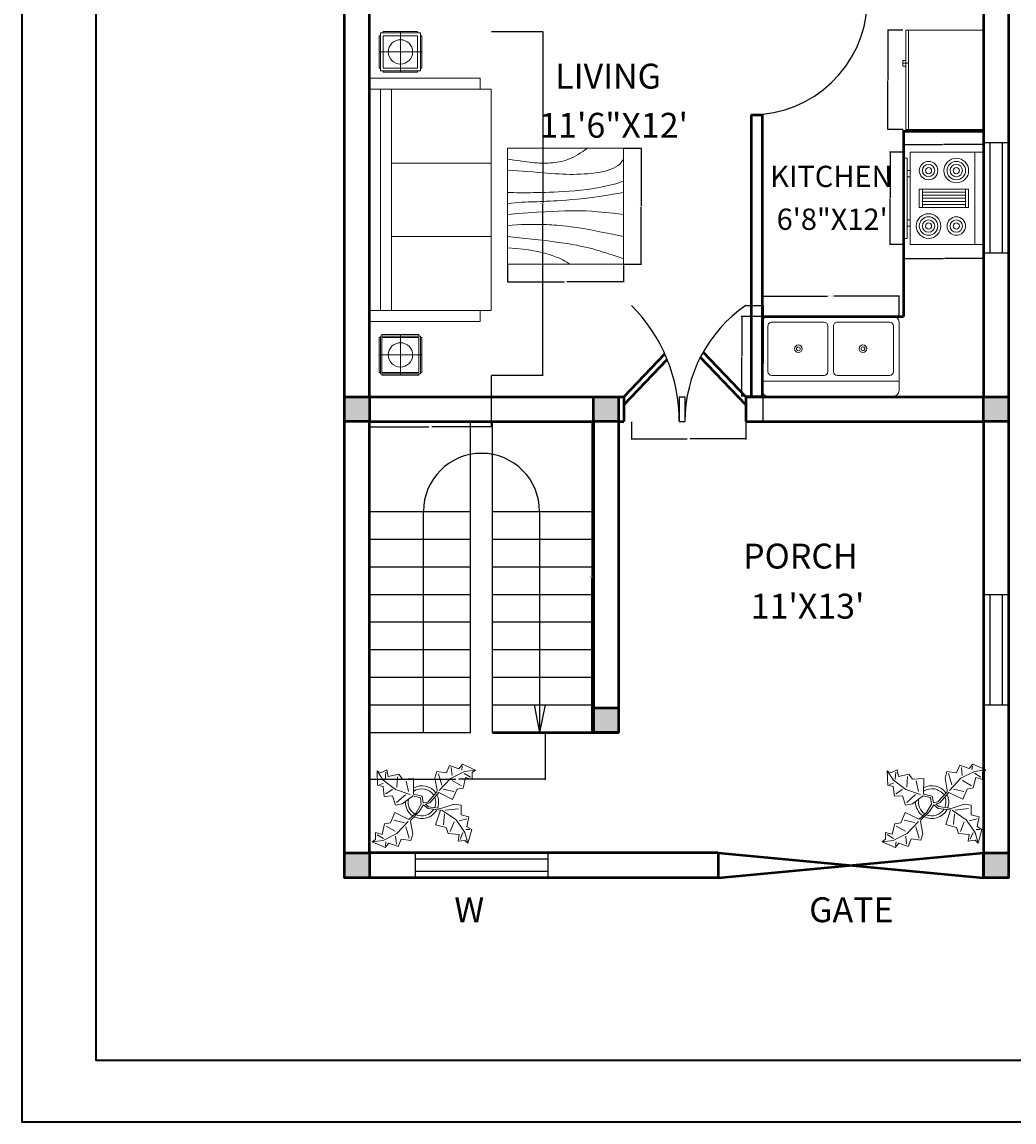
# Model space of a CAD drawing. Units: inches. Extents: x 28637 to 29820, y 17246 to 17928.
# Tile 1 of 6: x 28637 to 28996, y 17246 to 17644. Entities that reach past the tile are written whole.
import ezdxf

# ---------------------------------------------------------------- set-up
doc = ezdxf.new("R2010")
doc.units = ezdxf.units.IN
for name, color, linetype, lineweight in [('A-ANNO-DIMS', 2, 'Continuous', 18), ('A-ANNO-TEXT', 7, 'Continuous', 25), ('A-ANNO-TTLB', 7, 'Continuous', 35), ('A-AREA-IDEN', 30, 'Continuous', 25), ('A-COLS', 1, 'Continuous', 50), ('A-DOOR', 4, 'Continuous', 25), ('A-FLOR-FIXT', 8, 'Continuous', 18), ('A-FLOR-STRS', 3, 'Continuous', 25), ('A-FURN', 8, 'Continuous', 18), ('A-GLAZ', 4, 'Continuous', 25), ('A-WALL', 7, 'Continuous', 50)]:
    doc.layers.add(name, color=color, linetype=linetype, lineweight=lineweight)
doc.styles.get("Standard").update_dxf_attribs({"font": 'arial.ttf'})
doc.dimstyles.get("Standard").update_dxf_attribs({"dimtxt": 0.18, "dimasz": 0.18, "dimexe": 0.18, "dimexo": 0.0625, "dimgap": 0.09, "dimtad": 0, "dimtih": 1, "dimtoh": 1, "dimdec": 4, "dimzin": 0, "dimdsep": 46, "dimtxsty": 'Standard', "dimcen": 0.09, "dimadec": 0, "dimazin": 0, "dimtfac": 1, "dimtdec": 4, "dimtofl": 0, "dimtmove": 0, "dimatfit": 3, "dimfxl": 1, "dimtolj": 1, "dimtzin": 0, "dimarcsym": 0})

# ---------------------------------------------------------------- blocks, each defined once
blk = doc.blocks.new('Range-Oven - 30 in top')
for p, q in [((0, -3), (30, -3)), ((12, -6), (18, -6)), ((13, -20), (13, -6)), ((14, -6), (14, -20)), ((15, -20), (15, -6)), ((16, -6), (16, -20)), ((17, -20), (17, -6)), ((18, -20), (12, -20)), ((6, -24), (6, -25)), ((8, -25), (8, -24)), ((22, -25), (22, -24)), ((24, -24), (24, -25))]:
    blk.add_line(p, q)
for points in [[(0, -24), (0, 0), (30, 0), (30, -24)], [(12, -21), (12, -5), (18, -5), (18, -21)], [(2, -26), (2, -25), (28, -25), (28, -26)]]:
    blk.add_lwpolyline(points, close=True)
for centre, radius in [((6, -9), 4), ((6, -9), 3), ((6, -9), 2), ((24, -9), 3), ((24, -9), 2), ((6, -9), 1), ((24, -9), 1), ((24, -18), 4), ((6, -18), 3), ((6, -18), 2), ((6, -18), 1), ((24, -18), 3), ((24, -18), 2), ((24, -18), 1)]:
    blk.add_circle(centre, radius)
blk = doc.blocks.new('Refrigerator-2 door - 36 in top')
for p, q in [((0, -26.999999), (36, -26.999999)), ((12, -26.999999), (12, -28.999999)), ((11, -27.999999), (11, -28.999999)), ((11, -28.999999), (13, -28.999999)), ((13, -28.999999), (13, -27.999999))]:
    blk.add_line(p, q)
blk.add_lwpolyline([(0, -27.999999), (0, 0), (36, 0), (36, -27.999999)], close=True)
blk = doc.blocks.new('Sink-double - 36 in top')
for p, q in [((-18, -4), (18, -4)), ((-0.75, -18.5), (-0.75, -6.5)), ((0.75, -6.5), (0.75, -18.5))]:
    blk.add_line(p, q)
for points in [[(-16.5, 0), (16.5, 0)], [(-18, -19.5), (-18, -1.5)], [(18, -1.5), (18, -19.5)], [(-15.5, -5.5), (-1.75, -5.5)], [(1.75, -5.5), (15.5, -5.5)], [(-16.5, -18.5), (-16.5, -6.5)], [(16.5, -6.5), (16.5, -18.5)], [(-1.75, -19.5), (-15.5, -19.5)], [(15.5, -19.5), (1.75, -19.5)], [(16.5, -21), (-16.5, -21)]]:
    blk.add_lwpolyline(points)
for centre, radius in [((-8.5, -12.5), 1), ((8.5, -12.5), 1), ((-8.5, -12.5), 0.5), ((8.5, -12.5), 0.5)]:
    blk.add_circle(centre, radius)
for centre, radius, start, end in [((-16.5, -1.5), 1.5, 90, 180), ((16.5, -1.5), 1.5, 0, 90), ((-15.5, -6.5), 1, 90, 180), ((-1.75, -6.5), 1, 0, 90), ((1.75, -6.5), 1, 90, 180), ((15.5, -6.5), 1, 0, 90), ((-16.5, -19.5), 1.5, 180, 270), ((-15.5, -18.5), 1, 180, 270), ((-1.75, -18.5), 1, 270, 0), ((1.75, -18.5), 1, 180, 270), ((15.5, -18.5), 1, 270, 0), ((16.5, -19.5), 1.5, 270, 0)]:
    blk.add_arc(centre, radius, start, end)
blk = doc.blocks.new('Table - Square Woodgrain 42 x 42 in.')
blk.add_line((0, -42), (42, -42))
for points in [[(0, -4), (1.704, -4.2172), (3.2358, -4.4188), (4.615, -4.604), (5.8615, -4.7721), (6.9951, -4.9224), (8.0357, -5.0541), (9.0031, -5.1667), (9.9171, -5.2594), (10.7951, -5.3316), (11.6445, -5.3836), (12.4702, -5.4157), (13.277, -5.4283), (14.0698, -5.4217), (14.8535, -5.3964), (15.6331, -5.3526), (16.4133, -5.2908), (17.1986, -5.2103), (17.9913, -5.1062), (18.793, -4.9727), (19.6056, -4.8038), (20.4307, -4.5937), (21.2701, -4.3365), (22.1256, -4.0262), (22.9989, -3.6571), (23.888, -3.2272), (24.7756, -2.7516), (25.6408, -2.2491), (26.4624, -1.7387), (27.2195, -1.2395), (27.891, -0.7703), (28.456, -0.3501), (28.8934, 0.002)], [(0, -42), (0, 0), (42, 0), (42, -42)], [(0, -8), (1.8203, -8.1001), (3.6741, -8.2149), (5.5411, -8.3408), (7.4011, -8.4741), (9.2339, -8.6112), (11.0193, -8.7484), (12.7371, -8.8821), (14.3671, -9.0086), (15.8954, -9.1246), (17.3337, -9.2278), (18.6997, -9.3159), (20.0116, -9.387), (21.2871, -9.4389), (22.5442, -9.4696), (23.8008, -9.477), (25.0749, -9.459), (26.3791, -9.4137), (27.7049, -9.3403), (29.0383, -9.2382), (30.3655, -9.1068), (31.6728, -8.9455), (32.9461, -8.7535), (34.1717, -8.5304), (35.3358, -8.2756), (36.4268, -7.9863), (37.443, -7.6521), (38.3849, -7.2603), (39.253, -6.7986), (40.048, -6.2542), (40.7705, -5.6147), (41.421, -4.8674), (42, -4)], [(42, -12), (39.1784, -12.8621), (36.4519, -13.5654), (33.8246, -14.1294), (31.3004, -14.5731), (28.8832, -14.9161), (26.577, -15.1775), (24.3858, -15.3768), (22.3136, -15.5332), (20.3622, -15.6632), (18.5254, -15.7718), (16.7947, -15.8612), (15.1618, -15.9338), (13.6183, -15.9916), (12.1558, -16.0369), (10.7659, -16.0718), (9.4403, -16.0987), (8.1703, -16.1191), (6.9461, -16.1325), (5.7577, -16.1377), (4.595, -16.1335), (3.4479, -16.1188), (2.3064, -16.0924), (1.1604, -16.0532), (0, -16)], [(42, -16), (37.6529, -16.7365), (33.8802, -17.329), (30.6179, -17.7961), (27.8015, -18.1561), (25.3668, -18.4275), (23.2497, -18.6288), (21.3859, -18.7785), (19.7111, -18.8949), (18.1693, -18.9939), (16.7375, -19.0795), (15.401, -19.1534), (14.1449, -19.217), (12.9544, -19.2717), (11.8148, -19.3191), (10.7113, -19.3606), (9.6291, -19.3976), (8.5534, -19.4323), (7.47, -19.4689), (6.3643, -19.5122), (5.222, -19.5672), (4.0288, -19.6386), (2.7703, -19.7313), (1.4321, -19.8501), (0, -20)], [(0, -24), (3.9243, -23.6805), (7.4766, -23.4138), (10.6891, -23.1954), (13.5943, -23.0205), (16.2247, -22.8847), (18.6125, -22.7832), (20.7903, -22.7116), (22.7903, -22.6651), (24.6563, -22.642), (26.4764, -22.6507), (28.35, -22.7024), (30.3766, -22.8084), (32.6555, -22.98), (35.2861, -23.2283), (38.3678, -23.5645), (42, -24)], [(42, -32), (37.392, -31.017), (33.4585, -30.2231), (30.1291, -29.5949), (27.3334, -29.109), (25.0009, -28.742), (23.0612, -28.4707), (21.4439, -28.2716), (20.0786, -28.1215), (18.8998, -28.0002), (17.8609, -27.9014), (16.9206, -27.8219), (16.0371, -27.7588), (15.1691, -27.709), (14.2748, -27.6693), (13.3128, -27.6368), (12.2415, -27.6083), (11.0295, -27.5824), (9.6867, -27.5643), (8.233, -27.5608), (6.6884, -27.5787), (5.0728, -27.6248), (3.4062, -27.7058), (1.7086, -27.8286), (0, -28)], [(0, -32), (5.4026, -32.5358), (9.9494, -33.019), (13.7424, -33.4553), (16.8834, -33.8505), (19.4743, -34.2106), (21.6171, -34.5413), (23.4136, -34.8486), (24.9657, -35.1382), (26.3614, -35.4156), (27.6332, -35.6841), (28.7995, -35.9467), (29.8788, -36.2064), (30.8897, -36.4661), (31.8507, -36.7288), (32.7802, -36.9973), (33.6968, -37.2747), (34.6175, -37.5635), (35.5531, -37.8651), (36.5128, -38.1805), (37.506, -38.5108), (38.5421, -38.8568), (39.6302, -39.2197), (40.7797, -39.6004), (42, -40)], [(0, -36), (3.0098, -36.2857), (5.5354, -36.5643), (7.6368, -36.8359), (9.374, -37.1009), (10.807, -37.3597), (11.9957, -37.6126), (13.0002, -37.8599), (13.8804, -38.102), (14.6874, -38.3393), (15.4365, -38.5729), (16.1338, -38.8041), (16.7858, -39.0341), (17.3987, -39.264), (17.9787, -39.4952), (18.5322, -39.7288), (19.0655, -39.9662), (19.5832, -40.2081), (20.0842, -40.4544), (20.5657, -40.7046), (21.0249, -40.9581), (21.459, -41.2144), (21.8653, -41.4731), (22.2409, -41.7335), (22.5831, -41.9951)]]:
    blk.add_lwpolyline(points)
blk = doc.blocks.new('Plant - Rubber or Philodendron')
for p, q in [((8.8871, 10.7908), (9.9809, 13.4933)), ((9.9809, 13.4933), (13.3837, 12.301)), ((10.5828, 12.6946), (10.8893, 9.7953)), ((13.3837, 12.301), (14.68, 13.9039)), ((14.5816, 13.2037), (14.3848, 11.8033)), ((14.68, 13.9039), (19.3848, 11.8146)), ((-16.2005, 11.4774), (-13.9899, 8.1064)), ((-16.2005, 11.4774), (-14.8639, 10.7964)), ((-16.0159, 6.3329), (-16.2005, 11.4774)), ((-14.8639, 10.7964), (-12.6195, 11.8975)), ((-13.9899, 8.1064), (-9.5434, 4.7185)), ((-13.3174, 8.325), (-13.0735, 11.0065)), ((-12.6195, 11.8975), (-12.1909, 9.4345)), ((-12.1909, 9.4345), (-8.3829, 10.3)), ((-8.8369, 9.409), (-9.0894, 5.6095)), ((-8.3829, 10.3), (-7.0549, 8.501)), ((-7.0549, 8.501), (-3.0284, 8.6941)), ((-3.0284, 8.6941), (-3.0709, 3.1041)), ((4.6914, 8.8812), (5.3859, 11.2828)), ((4.6914, 8.8812), (5.5014, 4.4831)), ((5.3859, 11.2828), (8.8871, 10.7908)), ((5.9878, 10.4842), (7.1971, 6.3869)), ((10.3916, 8.7942), (6.2847, 4.4028)), ((15.3859, 11.3055), (10.3916, 8.7942)), ((14.2977, 6.1031), (10.9934, 7.9956)), ((15.7909, 9.1065), (14.8995, 5.3044)), ((15.2875, 10.6053), (17.5907, 9.2105)), ((19.3848, 11.8146), (15.3859, 11.3055)), ((18.1925, 8.4119), (15.7909, 9.1065)), ((19.3848, 11.8146), (18.1868, 10.9119)), ((18.1868, 10.9119), (18.1925, 8.4119)), ((-14.0069, 5.8704), (-16.0159, 6.3329)), ((-15.3434, 6.5514), (-13.9984, 6.9884)), ((-13.5868, 2.2894), (-14.0069, 5.8704)), ((-13.1329, 3.1804), (-10.6614, 4.727)), ((-9.5434, 4.7185), (-4.1917, 2.9888)), ((-4.8529, 4.012), (-5.7184, 7.82)), ((5.4346, 3.9146), (5.5014, 4.4831)), ((7.7005, 4.8881), (11.5025, 3.9967)), ((12.7005, 4.8994), (11.1089, 1.1958)), ((14.8995, 5.3044), (12.7005, 4.8994)), ((-10.6784, 2.491), (-13.5868, 2.2894)), ((-9.5858, -0.8715), (-10.6784, 2.491)), ((-9.1318, 0.0195), (-5.9793, 2.9025)), ((-7.1228, -0.443), (-3.5248, 2.2131)), ((-3.5248, 2.2131), (-3.3011, 2.4355)), ((-3.3011, 2.4355), (-0.5306, 1.7947)), ((-3.0709, 3.1041), (0.0797, 2.3163)), ((-0.5306, 1.7947), (-0.2255, -0.5527)), ((-0.5306, 1.7947), (-0.5306, 1.7947)), ((0.0797, 2.3163), (0.4866, -0.031)), ((0.4866, -0.031), (2.1141, 0.2298)), ((2.1141, 0.2298), (5.4346, 3.9146)), ((6.1032, 3.6844), (2.8262, -0.031)), ((11.1089, 1.1958), (6.1032, 3.6844)), ((-11.3237, -7.2629), (-9.7321, -3.5593)), ((-9.7321, -3.5593), (-4.7264, -6.0479)), ((-7.1228, -0.443), (-9.5858, -0.8715)), ((-2.019, -3.6148), (-4.7264, -6.0479)), ((-4.0579, -6.2781), (-0.9375, -3.1608)), ((-2.019, -3.6148), (-0.2255, -0.5527)), ((-0.9375, -3.1608), (0.5883, -0.8135)), ((0.5883, -0.8135), (2.2447, -2.0916)), ((2.8262, -0.031), (1.3003, -0.5527)), ((1.3003, -0.5527), (2.4193, -1.4655)), ((2.2447, -2.0916), (6.7108, -2.6626)), ((2.4193, -1.4655), (6.895, -2.1175)), ((4.943, -7.9659), (6.7108, -2.6626)), ((11.6605, -0.5413), (6.895, -2.1175)), ((12.3677, -6.1981), (7.219, -2.6772)), ((8.3544, -2.7453), (13.1973, -2.1704)), ((11.6605, -0.5413), (14.1354, -0.8948)), ((14.1354, -0.8948), (14.1354, -4.4304)), ((-14.4141, -11.4699), (-13.5228, -7.6679)), ((-13.5228, -7.6679), (-11.3237, -7.2629)), ((-6.3237, -7.2516), (-10.1257, -6.3602)), ((-9.0148, -11.1577), (-4.9047, -6.8122)), ((-4.1246, -6.8466), (-4.0579, -6.2781)), ((-3.3146, -11.2447), (-4.1246, -6.8466)), ((8.125, -4.0768), (7.7715, -7.9659)), ((10.2463, -10.4408), (11.6605, -6.9053)), ((15.5496, -10.7943), (12.3677, -6.1981)), ((16.2567, -5.8446), (13.4283, -6.5517)), ((14.1354, -4.4304), (16.9638, -5.1375)), ((16.9638, -5.1375), (16.2567, -8.673)), ((-16.8157, -10.7754), (-14.4141, -11.4699)), ((-16.8101, -13.2754), (-16.8157, -10.7754)), ((-13.9107, -12.9688), (-16.2139, -11.574)), ((-14.0091, -13.669), (-9.0148, -11.1577)), ((-12.921, -8.4665), (-9.6166, -10.359)), ((-4.611, -12.8477), (-5.8203, -8.7504)), ((-3.3146, -11.2447), (-4.0092, -13.6463)), ((8.8321, -9.0266), (4.943, -7.9659)), ((9.5392, -11.1479), (8.8321, -9.0266)), ((13.4283, -11.5015), (9.5392, -11.1479)), ((13.0748, -13.9763), (13.4283, -11.5015)), ((14.8425, -10.7943), (13.7819, -13.2692)), ((16.6103, -14.6834), (15.5496, -10.7943)), ((17.3174, -9.7337), (15.9032, -9.7337)), ((16.2567, -8.673), (18.0245, -9.7337)), ((18.0245, -9.7337), (16.6103, -14.6834)), ((-18.008, -14.1781), (-16.8101, -13.2754)), ((-18.008, -14.1781), (-14.0091, -13.669)), ((-13.3032, -16.2674), (-18.008, -14.1781)), ((-12.0069, -14.6645), (-13.3032, -16.2674)), ((-13.2048, -15.5672), (-13.008, -14.1668)), ((-8.6042, -15.8568), (-12.0069, -14.6645)), ((-9.206, -15.0581), (-9.5126, -12.1588)), ((-7.5103, -13.1543), (-8.6042, -15.8568)), ((-4.0092, -13.6463), (-7.5103, -13.1543)), ((15.5496, -13.6228), (13.0748, -13.9763)), ((16.6103, -14.6834), (15.5496, -13.6228))]:
    blk.add_line(p, q)
for centre, radius, start, end in [((0, 0), 6.1275, 34.37569, 120.1028), ((-0.0601, -0.2075), 5.2461, 33.82192, 124.9414), ((0.0308, 0.1664), 6, 178.6147, 235.1169), ((0.0308, 0.1664), 5, 168.1647, 238.6725), ((-0.2664, 0.1682), 5.2775, 338.4094, 20.03007), ((-0.098, 0.1364), 6.1288, 341.2017, 26.09184), ((-0.0234, 0.3825), 6.1492, 242.5812, 331.2714), ((-0.1102, 0.4886), 5.2883, 247.3711, 327.472)]:
    blk.add_arc(centre, radius, start, end)
blk = doc.blocks.new('DOOR-42')
blk.add_line((28900.64, 17650.75), (28942.64, 17650.75))
blk.add_arc((28900.64, 17652.8), 42.05, 270, 357.2056)
blk = doc.blocks.new('DOOR-DOUBLE')
for p, q in [((17.27, 9), (17.27, 0)), ((17.27, 9), (19.27, 9)), ((19.27, 9), (19.27, 0)), ((19.27, 9), (19.27, 0)), ((17.27, 0), (19.27, 0))]:
    blk.add_line(p, q)
for centre, radius, start, end in [((-42.45, 0), 59.72, 0, 44.6951), ((70.36, 0), 51.09, 124.708, 180)]:
    blk.add_arc(centre, radius, start, end)
blk = doc.blocks.new('STAIR')
for p, q in [((28799.14, 17387.25), (28799.14, 17499.75)), ((28807.14, 17387.25), (28807.14, 17499.75)), ((28762.64, 17467.25), (28799.14, 17467.25)), ((28782.14, 17387.25), (28782.14, 17467.25)), ((28824.14, 17467.25), (28824.14, 17387.25)), ((28762.64, 17457.25), (28799.14, 17457.25)), ((28762.64, 17447.25), (28799.14, 17447.25)), ((28762.64, 17437.25), (28799.14, 17437.25)), ((28762.64, 17427.25), (28799.14, 17427.25)), ((28762.64, 17417.25), (28799.14, 17417.25)), ((28762.64, 17407.25), (28799.14, 17407.25)), ((28762.64, 17397.25), (28799.14, 17397.25)), ((28822.14, 17397.25), (28824.14, 17387.25)), ((28826.14, 17397.25), (28824.14, 17387.25)), ((28762.64, 17387.25), (28799.14, 17387.25))]:
    blk.add_line(p, q)
blk.add_arc((28803.14, 17467.25), 21, 0, 180)
blk = doc.blocks.new('SOFA-SET')
for p, q in [((28780.04, 17640.82), (28767.64, 17640.82)), ((28767.64, 17640.32), (28767.64, 17640.82)), ((28773.84, 17640.82), (28773.84, 17626.13)), ((28780.04, 17640.32), (28780.04, 17640.82)), ((28766.64, 17639.32), (28766.14, 17639.32)), ((28766.14, 17639.32), (28766.14, 17627.63)), ((28781.04, 17639.32), (28781.54, 17639.32)), ((28781.54, 17639.32), (28781.54, 17627.63)), ((28766.14, 17633.48), (28781.54, 17633.48)), ((28766.64, 17627.63), (28766.14, 17627.63)), ((28781.04, 17627.63), (28781.54, 17627.63)), ((28762.64, 17623.94), (28802.64, 17623.94)), ((28762.64, 17535.94), (28762.64, 17623.94)), ((28762.64, 17535.94), (28762.64, 17623.94)), ((28767.64, 17626.63), (28767.64, 17626.13)), ((28767.64, 17626.13), (28780.04, 17626.13)), ((28780.04, 17626.63), (28780.04, 17626.13)), ((28802.64, 17619.94), (28802.64, 17623.94)), ((28762.64, 17619.94), (28806.64, 17619.94)), ((28766.64, 17539.94), (28766.64, 17619.94)), ((28770.64, 17539.94), (28770.64, 17619.94)), ((28806.64, 17539.94), (28806.64, 17619.94)), ((28770.64, 17593.24), (28806.64, 17593.24)), ((28770.64, 17566.64), (28806.64, 17566.64)), ((28762.64, 17539.94), (28806.64, 17539.94)), ((28802.64, 17535.94), (28802.64, 17539.94)), ((28762.64, 17535.94), (28802.64, 17535.94)), ((28766.64, 17530.2), (28766.14, 17530.2)), ((28766.14, 17530.2), (28766.14, 17517.52)), ((28767.14, 17530.7), (28767.14, 17531.2)), ((28767.14, 17531.2), (28780.54, 17531.2)), ((28773.84, 17516.52), (28773.84, 17531.2)), ((28780.54, 17530.7), (28780.54, 17531.2)), ((28781.04, 17530.2), (28781.54, 17530.2)), ((28781.54, 17530.2), (28781.54, 17517.52)), ((28766.14, 17523.86), (28781.54, 17523.86)), ((28766.64, 17517.52), (28766.14, 17517.52)), ((28767.14, 17517.02), (28767.14, 17516.52)), ((28780.54, 17516.52), (28767.14, 17516.52)), ((28780.54, 17517.02), (28780.54, 17516.52)), ((28781.04, 17517.52), (28781.54, 17517.52))]:
    blk.add_line(p, q)
for points in [[(28766.64, 17640.32), (28781.04, 17640.32), (28781.04, 17626.63), (28766.64, 17626.63)], [(28767.64, 17639.32), (28780.04, 17639.32), (28780.04, 17627.63), (28767.64, 17627.63)], [(28766.64, 17530.7), (28781.04, 17530.7), (28781.04, 17517.02), (28766.64, 17517.02)], [(28767.14, 17530.2), (28780.54, 17530.2), (28780.54, 17517.52), (28767.14, 17517.52)]]:
    blk.add_lwpolyline(points, close=True)
for centre in [(28773.84, 17633.48), (28773.84, 17523.86)]:
    blk.add_circle(centre, 4.4)
blk = doc.blocks.new('*D42')
at = {"layer": 'A-ANNO-DIMS', "color": 0, "lineweight": -2, "transparency": 16777216}
for p, q in [((28898.71, 17541.75), (28905.12, 17541.75)), ((28904.94, 17541.57), (28904.94, 17520.94)), ((28904.94, 17499.93), (28904.94, 17520.57)), ((28898.71, 17499.75), (28905.12, 17499.75))]:
    blk.add_line(p, q, dxfattribs=at)
at = {"layer": 'A-ANNO-DIMS', "color": 0, "transparency": 16777216}
for points in [[(28904.91, 17541.57), (28904.97, 17541.57), (28904.94, 17541.75)], [(28904.91, 17499.93), (28904.97, 17499.93), (28904.94, 17499.75)]]:
    blk.add_solid(points, dxfattribs=at)
at = {"layer": 'Defpoints', "color": 0, "transparency": 16777216}
for p in [(28898.64, 17541.75), (28904.94, 17541.75), (28898.64, 17499.75)]:
    blk.add_point(p, dxfattribs=at)
at = {"layer": 'A-ANNO-DIMS', "color": 0, "transparency": 16777216, "insert": (28904.94, 17520.75), "char_height": 0.18, "attachment_point": 5}
blk.add_mtext('\\A1;DOUBLE DOOR 42 TYP.', dxfattribs=at)
blk = doc.blocks.new('*D43')
at = {"layer": 'A-ANNO-DIMS', "color": 0, "lineweight": -2, "transparency": 16777216}
for p, q in [((28857.38, 17499.69), (28857.38, 17493.27)), ((28898.64, 17499.69), (28898.64, 17493.27)), ((28857.56, 17493.45), (28877.48, 17493.45)), ((28898.46, 17493.45), (28878.54, 17493.45))]:
    blk.add_line(p, q, dxfattribs=at)
at = {"layer": 'A-ANNO-DIMS', "color": 0, "transparency": 16777216}
for points in [[(28857.56, 17493.48), (28857.56, 17493.42), (28857.38, 17493.45)], [(28898.46, 17493.48), (28898.46, 17493.42), (28898.64, 17493.45)]]:
    blk.add_solid(points, dxfattribs=at)
at = {"layer": 'Defpoints', "color": 0, "transparency": 16777216}
for p in [(28857.38, 17499.75), (28898.64, 17499.75), (28898.64, 17493.45)]:
    blk.add_point(p, dxfattribs=at)
at = {"layer": 'A-ANNO-DIMS', "color": 0, "transparency": 16777216, "insert": (28878.01, 17493.45), "char_height": 0.18, "attachment_point": 5}
blk.add_mtext('\\A1;41 TYP.', dxfattribs=at)
blk = doc.blocks.new('*D44')
at = {"layer": 'A-ANNO-DIMS', "color": 0, "lineweight": -2, "transparency": 16777216}
for p, q in [((28826.21, 17499.75), (28843.2, 17499.75)), ((28843.02, 17499.57), (28843.02, 17443.69)), ((28843.02, 17387.43), (28843.02, 17443.32)), ((28826.21, 17387.25), (28843.2, 17387.25))]:
    blk.add_line(p, q, dxfattribs=at)
at = {"layer": 'A-ANNO-DIMS', "color": 0, "transparency": 16777216}
for points in [[(28842.99, 17499.57), (28843.05, 17499.57), (28843.02, 17499.75)], [(28842.99, 17387.43), (28843.05, 17387.43), (28843.02, 17387.25)]]:
    blk.add_solid(points, dxfattribs=at)
at = {"layer": 'Defpoints', "color": 0, "transparency": 16777216}
for p in [(28826.14, 17499.75), (28843.02, 17499.75), (28826.14, 17387.25)]:
    blk.add_point(p, dxfattribs=at)
at = {"layer": 'A-ANNO-DIMS', "color": 0, "transparency": 16777216, "insert": (28843.02, 17443.5), "char_height": 0.18, "attachment_point": 5}
blk.add_mtext('\\A1;STAIR 113 TYP.', dxfattribs=at)
blk = doc.blocks.new('*D45')
at = {"layer": 'A-ANNO-DIMS', "color": 0, "lineweight": -2, "transparency": 16777216}
for p, q in [((28762.64, 17387.19), (28762.64, 17370.2)), ((28826.14, 17387.19), (28826.14, 17370.2)), ((28762.82, 17370.38), (28793.87, 17370.38)), ((28825.96, 17370.38), (28794.92, 17370.38))]:
    blk.add_line(p, q, dxfattribs=at)
at = {"layer": 'A-ANNO-DIMS', "color": 0, "transparency": 16777216}
for points in [[(28762.82, 17370.41), (28762.82, 17370.35), (28762.64, 17370.38)], [(28825.96, 17370.41), (28825.96, 17370.35), (28826.14, 17370.38)]]:
    blk.add_solid(points, dxfattribs=at)
at = {"layer": 'Defpoints', "color": 0, "transparency": 16777216}
for p in [(28762.64, 17387.25), (28826.14, 17387.25), (28826.14, 17370.38)]:
    blk.add_point(p, dxfattribs=at)
at = {"layer": 'A-ANNO-DIMS', "color": 0, "transparency": 16777216, "insert": (28794.39, 17370.38), "char_height": 0.18, "attachment_point": 5}
blk.add_mtext('\\A1;64 TYP.', dxfattribs=at)
blk = doc.blocks.new('*D46')
at = {"layer": 'A-ANNO-DIMS', "color": 0, "lineweight": -2, "transparency": 16777216}
for p, q in [((28806.71, 17640.82), (28825.47, 17640.82)), ((28825.29, 17640.64), (28825.29, 17578.85)), ((28825.29, 17516.7), (28825.29, 17578.49)), ((28806.71, 17516.52), (28825.47, 17516.52))]:
    blk.add_line(p, q, dxfattribs=at)
at = {"layer": 'A-ANNO-DIMS', "color": 0, "transparency": 16777216}
for points in [[(28825.26, 17640.64), (28825.32, 17640.64), (28825.29, 17640.82)], [(28825.26, 17516.7), (28825.32, 17516.7), (28825.29, 17516.52)]]:
    blk.add_solid(points, dxfattribs=at)
at = {"layer": 'Defpoints', "color": 0, "transparency": 16777216}
for p in [(28806.64, 17640.82), (28825.29, 17640.82), (28806.64, 17516.52)]:
    blk.add_point(p, dxfattribs=at)
at = {"layer": 'A-ANNO-DIMS', "color": 0, "transparency": 16777216, "insert": (28825.29, 17578.67), "char_height": 0.18, "attachment_point": 5}
blk.add_mtext('\\A1;SOFA SET 124 TYP.', dxfattribs=at)
blk = doc.blocks.new('*D47')
at = {"layer": 'A-ANNO-DIMS', "color": 0, "lineweight": -2, "transparency": 16777216}
for p, q in [((28762.64, 17516.45), (28762.64, 17497.69)), ((28806.64, 17516.45), (28806.64, 17497.69)), ((28762.82, 17497.87), (28784.11, 17497.87)), ((28806.46, 17497.87), (28785.18, 17497.87))]:
    blk.add_line(p, q, dxfattribs=at)
at = {"layer": 'A-ANNO-DIMS', "color": 0, "transparency": 16777216}
for points in [[(28762.82, 17497.9), (28762.82, 17497.84), (28762.64, 17497.87)], [(28806.46, 17497.9), (28806.46, 17497.84), (28806.64, 17497.87)]]:
    blk.add_solid(points, dxfattribs=at)
at = {"layer": 'Defpoints', "color": 0, "transparency": 16777216}
for p in [(28762.64, 17516.52), (28806.64, 17516.52), (28806.64, 17497.87)]:
    blk.add_point(p, dxfattribs=at)
at = {"layer": 'A-ANNO-DIMS', "color": 0, "transparency": 16777216, "insert": (28784.64, 17497.87), "char_height": 0.18, "attachment_point": 5}
blk.add_mtext('\\A1;44 TYP.', dxfattribs=at)
blk = doc.blocks.new('*D48')
at = {"layer": 'A-ANNO-DIMS', "color": 0, "lineweight": -2, "transparency": 16777216}
for p, q in [((28854.56, 17598.65), (28860.98, 17598.65)), ((28860.8, 17598.47), (28860.8, 17577.84)), ((28860.8, 17556.83), (28860.8, 17577.47)), ((28854.56, 17556.65), (28860.98, 17556.65))]:
    blk.add_line(p, q, dxfattribs=at)
at = {"layer": 'A-ANNO-DIMS', "color": 0, "transparency": 16777216}
for points in [[(28860.77, 17598.47), (28860.83, 17598.47), (28860.8, 17598.65)], [(28860.77, 17556.83), (28860.83, 17556.83), (28860.8, 17556.65)]]:
    blk.add_solid(points, dxfattribs=at)
at = {"layer": 'Defpoints', "color": 0, "transparency": 16777216}
for p in [(28854.5, 17598.65), (28860.8, 17598.65), (28854.5, 17556.65)]:
    blk.add_point(p, dxfattribs=at)
at = {"layer": 'A-ANNO-DIMS', "color": 0, "transparency": 16777216, "insert": (28860.8, 17577.65), "char_height": 0.18, "attachment_point": 5}
blk.add_mtext('\\A1;CENTER TABLE 42 TYP.', dxfattribs=at)
blk = doc.blocks.new('*D49')
at = {"layer": 'A-ANNO-DIMS', "color": 0, "lineweight": -2, "transparency": 16777216}
for p, q in [((28812.5, 17556.59), (28812.5, 17550.17)), ((28854.5, 17556.59), (28854.5, 17550.17)), ((28812.68, 17550.35), (28832.97, 17550.35)), ((28854.32, 17550.35), (28834.03, 17550.35))]:
    blk.add_line(p, q, dxfattribs=at)
at = {"layer": 'A-ANNO-DIMS', "color": 0, "transparency": 16777216}
for points in [[(28812.68, 17550.38), (28812.68, 17550.32), (28812.5, 17550.35)], [(28854.32, 17550.38), (28854.32, 17550.32), (28854.5, 17550.35)]]:
    blk.add_solid(points, dxfattribs=at)
at = {"layer": 'Defpoints', "color": 0, "transparency": 16777216}
for p in [(28812.5, 17556.65), (28854.5, 17556.65), (28854.5, 17550.35)]:
    blk.add_point(p, dxfattribs=at)
at = {"layer": 'A-ANNO-DIMS', "color": 0, "transparency": 16777216, "insert": (28833.5, 17550.35), "char_height": 0.18, "attachment_point": 5}
blk.add_mtext('\\A1;42 TYP.', dxfattribs=at)
blk = doc.blocks.new('*D54')
at = {"layer": 'A-ANNO-DIMS', "color": 0, "lineweight": -2, "transparency": 16777216}
for p, q in [((28955.78, 17597.22), (28950.65, 17597.22)), ((28950.83, 17597.04), (28950.83, 17580.69)), ((28950.83, 17563.97), (28950.83, 17580.32)), ((28955.78, 17563.79), (28950.65, 17563.79))]:
    blk.add_line(p, q, dxfattribs=at)
at = {"layer": 'A-ANNO-DIMS', "color": 0, "transparency": 16777216}
for points in [[(28950.8, 17597.04), (28950.86, 17597.04), (28950.83, 17597.22)], [(28950.8, 17563.97), (28950.86, 17563.97), (28950.83, 17563.79)]]:
    blk.add_solid(points, dxfattribs=at)
at = {"layer": 'Defpoints', "color": 0, "transparency": 16777216}
for p in [(28955.85, 17597.22), (28950.83, 17563.79), (28955.85, 17563.79)]:
    blk.add_point(p, dxfattribs=at)
at = {"layer": 'A-ANNO-DIMS', "color": 0, "transparency": 16777216, "insert": (28950.83, 17580.51), "char_height": 0.18, "attachment_point": 5}
blk.add_mtext('\\A1;HOB 33', dxfattribs=at)
blk = doc.blocks.new('*D55')
at = {"layer": 'A-ANNO-DIMS', "color": 0, "lineweight": -2, "transparency": 16777216}
for p, q in [((28955.85, 17563.73), (28955.85, 17558.6)), ((28984.81, 17563.73), (28984.81, 17558.6)), ((28956.03, 17558.78), (28970.11, 17558.78)), ((28984.63, 17558.78), (28970.55, 17558.78))]:
    blk.add_line(p, q, dxfattribs=at)
at = {"layer": 'A-ANNO-DIMS', "color": 0, "transparency": 16777216}
for points in [[(28956.03, 17558.81), (28956.03, 17558.75), (28955.85, 17558.78)], [(28984.63, 17558.81), (28984.63, 17558.75), (28984.81, 17558.78)]]:
    blk.add_solid(points, dxfattribs=at)
at = {"layer": 'Defpoints', "color": 0, "transparency": 16777216}
for p in [(28955.85, 17563.79), (28984.81, 17563.79), (28984.81, 17558.78)]:
    blk.add_point(p, dxfattribs=at)
at = {"layer": 'A-ANNO-DIMS', "color": 0, "transparency": 16777216, "insert": (28970.33, 17558.78), "char_height": 0.18, "attachment_point": 5}
blk.add_mtext('\\A1;29', dxfattribs=at)
blk = doc.blocks.new('*D56')
at = {"layer": 'A-ANNO-DIMS', "color": 0, "lineweight": -2, "transparency": 16777216}
for p, q in [((28955.42, 17641.34), (28949.9, 17641.34)), ((28950.08, 17641.16), (28950.08, 17623.52)), ((28950.08, 17605.52), (28950.08, 17623.16)), ((28955.42, 17605.34), (28949.9, 17605.34))]:
    blk.add_line(p, q, dxfattribs=at)
at = {"layer": 'A-ANNO-DIMS', "color": 0, "transparency": 16777216}
for points in [[(28950.05, 17641.16), (28950.11, 17641.16), (28950.08, 17641.34)], [(28950.05, 17605.52), (28950.11, 17605.52), (28950.08, 17605.34)]]:
    blk.add_solid(points, dxfattribs=at)
at = {"layer": 'Defpoints', "color": 0, "transparency": 16777216}
for p in [(28955.48, 17641.34), (28950.08, 17605.34), (28955.48, 17605.34)]:
    blk.add_point(p, dxfattribs=at)
at = {"layer": 'A-ANNO-DIMS', "color": 0, "transparency": 16777216, "insert": (28950.08, 17623.34), "char_height": 0.18, "attachment_point": 5}
blk.add_mtext('\\A1;REFRIGERATOR 36', dxfattribs=at)
blk = doc.blocks.new('*D57')
at = {"layer": 'A-ANNO-DIMS', "color": 0, "lineweight": -2, "transparency": 16777216}
for p, q in [((28955.48, 17605.28), (28955.48, 17599.76)), ((28984.48, 17605.28), (28984.48, 17599.76)), ((28955.66, 17599.94), (28969.76, 17599.94)), ((28984.3, 17599.94), (28970.2, 17599.94))]:
    blk.add_line(p, q, dxfattribs=at)
at = {"layer": 'A-ANNO-DIMS', "color": 0, "transparency": 16777216}
for points in [[(28955.66, 17599.97), (28955.66, 17599.91), (28955.48, 17599.94)], [(28984.3, 17599.97), (28984.3, 17599.91), (28984.48, 17599.94)]]:
    blk.add_solid(points, dxfattribs=at)
at = {"layer": 'Defpoints', "color": 0, "transparency": 16777216}
for p in [(28955.48, 17605.34), (28984.48, 17605.34), (28984.48, 17599.94)]:
    blk.add_point(p, dxfattribs=at)
at = {"layer": 'A-ANNO-DIMS', "color": 0, "transparency": 16777216, "insert": (28969.98, 17599.94), "char_height": 0.18, "attachment_point": 5}
blk.add_mtext('\\A1;29', dxfattribs=at)
blk = doc.blocks.new('*D58')
at = {"layer": 'A-ANNO-DIMS', "color": 0, "lineweight": -2, "transparency": 16777216}
for p, q in [((28904.64, 17537.81), (28904.64, 17545.35)), ((28904.82, 17545.17), (28928.27, 17545.17)), ((28953.9, 17545.17), (28930.46, 17545.17)), ((28954.08, 17537.81), (28954.08, 17545.35))]:
    blk.add_line(p, q, dxfattribs=at)
at = {"layer": 'A-ANNO-DIMS', "color": 0, "transparency": 16777216}
for points in [[(28904.82, 17545.2), (28904.82, 17545.14), (28904.64, 17545.17)], [(28953.9, 17545.2), (28953.9, 17545.14), (28954.08, 17545.17)]]:
    blk.add_solid(points, dxfattribs=at)
at = {"layer": 'Defpoints', "color": 0, "transparency": 16777216}
for p in [(28904.64, 17545.17), (28904.64, 17537.75), (28954.08, 17537.75)]:
    blk.add_point(p, dxfattribs=at)
at = {"layer": 'A-ANNO-DIMS', "color": 0, "transparency": 16777216, "insert": (28929.36, 17545.17), "char_height": 0.18, "attachment_point": 5}
blk.add_mtext('\\A1;DOUBLE SINK 49', dxfattribs=at)
blk = doc.blocks.new('*D59')
at = {"layer": 'A-ANNO-DIMS', "color": 0, "lineweight": -2, "transparency": 16777216}
for p, q in [((28904.58, 17537.75), (28897.05, 17537.75)), ((28897.23, 17537.57), (28897.23, 17523.51)), ((28897.23, 17509.09), (28897.23, 17523.15)), ((28904.58, 17508.91), (28897.05, 17508.91))]:
    blk.add_line(p, q, dxfattribs=at)
at = {"layer": 'A-ANNO-DIMS', "color": 0, "transparency": 16777216}
for points in [[(28897.2, 17537.57), (28897.26, 17537.57), (28897.23, 17537.75)], [(28897.2, 17509.09), (28897.26, 17509.09), (28897.23, 17508.91)]]:
    blk.add_solid(points, dxfattribs=at)
at = {"layer": 'Defpoints', "color": 0, "transparency": 16777216}
for p in [(28904.64, 17537.75), (28897.23, 17508.91), (28904.64, 17508.91)]:
    blk.add_point(p, dxfattribs=at)
at = {"layer": 'A-ANNO-DIMS', "color": 0, "transparency": 16777216, "insert": (28897.23, 17523.33), "char_height": 0.18, "attachment_point": 5}
blk.add_mtext('\\A1;29', dxfattribs=at)

msp = doc.modelspace()

# ---------------------------------------------------------------- hatches: boundary and pattern name
at = {"layer": 'A-COLS'}
h = msp.add_hatch(color=256, dxfattribs=at)
h.dxf.hatch_style = 1
h.paths.add_polyline_path([(28753.64, 17508.75), (28753.64, 17499.75), (28762.64, 17499.75), (28762.64, 17508.75)])
h = msp.add_hatch(color=256, dxfattribs=at)
h.dxf.hatch_style = 1
h.paths.add_polyline_path([(28843.64, 17508.75), (28843.64, 17499.75), (28852.64, 17499.75), (28852.64, 17508.75)])
h = msp.add_hatch(color=256, dxfattribs=at)
h.dxf.hatch_style = 1
h.paths.add_polyline_path([(28984.64, 17508.75), (28984.64, 17499.75), (28993.64, 17499.75), (28993.64, 17508.75)])
h = msp.add_hatch(color=256, dxfattribs=at)
h.dxf.hatch_style = 1
h.paths.add_polyline_path([(28843.64, 17396.25), (28843.64, 17387.25), (28852.64, 17387.25), (28852.64, 17396.25)])
h = msp.add_hatch(color=256, dxfattribs=at)
h.dxf.hatch_style = 1
h.paths.add_polyline_path([(28753.64, 17343.75), (28753.64, 17334.75), (28762.64, 17334.75), (28762.64, 17343.75)])
h = msp.add_hatch(color=256, dxfattribs=at)
h.dxf.hatch_style = 1
h.paths.add_polyline_path([(28984.64, 17343.75), (28984.64, 17334.75), (28993.64, 17334.75), (28993.64, 17343.75)])

# ---------------------------------------------------------------- linework, layer by layer
at = {"layer": 'A-ANNO-TTLB'}
for points in [[(28637.03, 17927.97), (29820.02, 17927.97), (29820.02, 17246.37), (28637.03, 17246.37)], [(28663.78, 17907.18), (29794.75, 17907.18), (29794.75, 17268.65), (28663.78, 17268.65)]]:
    msp.add_lwpolyline(points, close=True, dxfattribs=at)
at = {"layer": 'A-COLS'}
for points in [[(28753.64, 17508.75), (28762.64, 17508.75), (28762.64, 17499.75), (28753.64, 17499.75)], [(28843.64, 17508.75), (28852.64, 17508.75), (28852.64, 17499.75), (28843.64, 17499.75)], [(28984.64, 17508.75), (28993.64, 17508.75), (28993.64, 17499.75), (28984.64, 17499.75)], [(28843.64, 17396.25), (28852.64, 17396.25), (28852.64, 17387.25), (28843.64, 17387.25)], [(28753.64, 17343.75), (28762.64, 17343.75), (28762.64, 17334.75), (28753.64, 17334.75)], [(28984.64, 17343.75), (28993.64, 17343.75), (28993.64, 17334.75), (28984.64, 17334.75)]]:
    msp.add_lwpolyline(points, close=True, dxfattribs=at)
at = {"layer": 'A-FLOR-STRS'}
for p, q in [((28807.14, 17467.25), (28843.64, 17467.25)), ((28807.14, 17457.25), (28843.64, 17457.25)), ((28807.14, 17447.25), (28843.64, 17447.25)), ((28807.14, 17437.25), (28843.64, 17437.25)), ((28807.14, 17427.25), (28843.64, 17427.25)), ((28807.14, 17417.25), (28843.64, 17417.25)), ((28807.14, 17407.25), (28843.64, 17407.25)), ((28807.14, 17397.25), (28843.64, 17397.25))]:
    msp.add_line(p, q, dxfattribs=at)
at = {"layer": 'A-GLAZ'}
for p, q in [((28984.64, 17600.75), (28993.64, 17600.75)), ((28986.89, 17600.75), (28986.89, 17560.75)), ((28991.39, 17600.75), (28991.39, 17560.75)), ((28984.64, 17560.75), (28993.64, 17560.75)), ((28984.64, 17437.25), (28993.64, 17437.25)), ((28986.89, 17437.25), (28986.89, 17397.25)), ((28991.39, 17437.25), (28991.39, 17397.25)), ((28984.64, 17397.25), (28993.64, 17397.25)), ((28779.14, 17343.75), (28779.14, 17334.75)), ((28827.14, 17341.5), (28779.14, 17341.5)), ((28827.14, 17343.75), (28827.14, 17334.75)), ((28827.14, 17337), (28779.14, 17337))]:
    msp.add_line(p, q, dxfattribs=at)
at = {"layer": 'A-WALL'}
for p, q in [((28753.64, 17334.75), (28753.64, 17814.75)), ((28993.64, 17814.75), (28993.64, 17334.75)), ((28762.64, 17508.75), (28762.64, 17652.75)), ((28984.64, 17652.75), (28984.64, 17508.75)), ((28900.64, 17610.75), (28904.64, 17610.75)), ((28900.64, 17610.75), (28900.64, 17508.75)), ((28904.64, 17610.75), (28904.64, 17508.75)), ((28955.64, 17604.75), (28955.64, 17537.75)), ((28955.64, 17604.75), (28984.64, 17604.75)), ((28904.64, 17537.75), (28955.64, 17537.75)), ((28854.64, 17508.75), (28869.42, 17524.19)), ((28898.64, 17508.75), (28883.24, 17524.85)), ((28854.64, 17505.86), (28870.27, 17522.19)), ((28898.64, 17505.86), (28882.24, 17523)), ((28762.64, 17508.75), (28854.64, 17508.75)), ((28854.64, 17508.75), (28854.64, 17499.75)), ((28898.64, 17508.75), (28984.64, 17508.75)), ((28898.64, 17508.75), (28898.64, 17499.75)), ((28898.64, 17508.75), (28900.64, 17508.75)), ((28762.64, 17343.75), (28762.64, 17499.75)), ((28762.64, 17499.75), (28843.64, 17499.75)), ((28843.64, 17499.75), (28843.64, 17387.25)), ((28852.64, 17499.75), (28852.64, 17387.25)), ((28852.64, 17499.75), (28854.64, 17499.75)), ((28898.64, 17499.75), (28984.64, 17499.75)), ((28984.64, 17499.75), (28984.64, 17334.75)), ((28807.14, 17387.25), (28852.64, 17387.25)), ((28888.64, 17343.75), (28762.64, 17343.75)), ((28843.64, 17343.75), (28762.64, 17343.75)), ((28888.64, 17343.75), (28888.64, 17334.75)), ((28888.64, 17343.75), (28984.64, 17334.75)), ((28888.64, 17334.75), (28984.64, 17343.75)), ((28888.64, 17334.75), (28753.64, 17334.75)), ((28993.64, 17334.75), (28984.64, 17334.75))]:
    msp.add_line(p, q, dxfattribs=at)

# ---------------------------------------------------------------- block references
at = {"layer": 'A-DOOR'}
for name, p in [('DOOR-42', (0, 0)), ('DOOR-DOUBLE', (28857.38, 17499.75))]:
    msp.add_blockref(name, p, dxfattribs=at)
at = {"layer": 'A-FLOR-FIXT', "rotation": 270}
msp.add_blockref('Refrigerator-2 door - 36 in top', (28984.48, 17641.34), dxfattribs=at)
at = {"layer": 'A-FLOR-FIXT'}
for name, p, xscale, yscale, zscale, rotation in [('Range-Oven - 30 in top', (28984.81, 17597.22), 1.114158809973933, 1.114158809973933, 1.114158809973933, 270), ('Sink-double - 36 in top', (28929.36, 17508.91), 1.373332452362471, 1.373332452362471, 1.373332452362471, 180)]:
    msp.add_blockref(name, p, dxfattribs=dict(at, xscale=xscale, yscale=yscale, zscale=zscale, rotation=rotation))
at = {"layer": 'A-FLOR-STRS'}
msp.add_blockref('STAIR', (0, 0), dxfattribs=at)
at = {"layer": 'A-FURN'}
for name, p in [('SOFA-SET', (0, 0)), ('Table - Square Woodgrain 42 x 42 in.', (28812.5, 17598.65)), ('Plant - Rubber or Philodendron', (28781.59, 17361.88)), ('Plant - Rubber or Philodendron', (28966.02, 17361.91))]:
    msp.add_blockref(name, p, dxfattribs=at)

# ---------------------------------------------------------------- texts
at = {"layer": 'A-ANNO-TEXT'}
for s, p in [('    W', (28782.31, 17318.65)), ('GATE', (28921.58, 17318.65))]:
    msp.add_text(s, height=9, dxfattribs=at).set_placement(p)
at = {"layer": 'A-AREA-IDEN'}
for s, height, p in [('LIVING', 9, (28829.77, 17620.2)), (' 11\'6"X12\'', 9, (28821.28, 17602.42)), ('KITCHEN', 7.696, (28907.48, 17584.58)), (' 6\'8"X12\'', 7.696, (28907.48, 17569.09)), ('PORCH', 9, (28897.71, 17446.58)), (" 11'X13'", 9, (28897.71, 17428.47))]:
    msp.add_text(s, height=height, dxfattribs=at).set_placement(p)

# ---------------------------------------------------------------- dimensions: what is measured, and where the dimension line sits
at = {"layer": 'A-ANNO-DIMS'}
for base, p1, p2, angle, text, picture, middle in [((28825.29, 17640.82), (28806.64, 17516.52), (28806.64, 17640.82), 90, 'SOFA SET <> TYP.', '*D46', (28825.29, 17578.67)), ((28950.08, 17605.34), (28955.48, 17641.34), (28955.48, 17605.34), 270, 'REFRIGERATOR <>', '*D56', (28950.08, 17623.34)), ((28860.8, 17598.65), (28854.5, 17556.65), (28854.5, 17598.65), 90, 'CENTER TABLE <> TYP.', '*D48', (28860.8, 17577.65)), ((28950.83, 17563.79), (28955.85, 17597.22), (28955.85, 17563.79), 270, 'HOB <>', '*D54', (28950.83, 17580.51)), ((28904.64, 17545.17), (28954.08, 17537.75), (28904.64, 17537.75), 180, 'DOUBLE SINK <>', '*D58', (28929.36, 17545.17)), ((28904.94, 17541.75), (28898.64, 17499.75), (28898.64, 17541.75), 90, 'DOUBLE DOOR <> TYP.', '*D42', (28904.94, 17520.75)), ((28843.01934626, 17499.75249242), (28826.14434626, 17387.25249242), (28826.14434626, 17499.75249242), 90, 'STAIR <> TYP.', '*D44', (28843.01934626, 17443.50249242))]:
    dim = msp.add_linear_dim(base=base, p1=p1, p2=p2, angle=angle, text=text, dimstyle='Standard', override={"dimdec": 0, "dimlfac": 1, "dimrnd": 0, "dimzin": 0, "dimdsep": 46, "dimlunit": 2}, dxfattribs=at)
    dim.commit()
    dim.dimension.update_dxf_attribs({"geometry": picture, "text_midpoint": middle})
for base, p1, p2, picture, middle in [((28984.48, 17599.94), (28955.48, 17605.34), (28984.48, 17605.34), '*D57', (28969.98, 17599.94)), ((28984.81, 17558.78), (28955.85, 17563.79), (28984.81, 17563.79), '*D55', (28970.33, 17558.78))]:
    dim = msp.add_linear_dim(base=base, p1=p1, p2=p2, dimstyle='Standard', override={"dimdec": 0, "dimlfac": 1, "dimrnd": 0, "dimzin": 0, "dimdsep": 46, "dimlunit": 2}, dxfattribs=at)
    dim.commit()
    dim.dimension.update_dxf_attribs({"geometry": picture, "text_midpoint": middle})
for base, p1, p2, picture, middle in [((28854.5, 17550.35), (28812.5, 17556.65), (28854.5, 17556.65), '*D49', (28833.5, 17550.35)), ((28806.64, 17497.87), (28762.64, 17516.52), (28806.64, 17516.52), '*D47', (28784.64, 17497.87)), ((28898.64, 17493.45), (28857.38, 17499.75), (28898.64, 17499.75), '*D43', (28878.01, 17493.45)), ((28826.14434626, 17370.37749242), (28762.64434626, 17387.25249242), (28826.14434626, 17387.25249242), '*D45', (28794.39434626, 17370.37749242))]:
    dim = msp.add_linear_dim(base=base, p1=p1, p2=p2, text='<> TYP.', dimstyle='Standard', override={"dimdec": 0, "dimlfac": 1, "dimrnd": 0, "dimzin": 0, "dimdsep": 46, "dimlunit": 2}, dxfattribs=at)
    dim.commit()
    dim.dimension.update_dxf_attribs({"geometry": picture, "text_midpoint": middle})
dim = msp.add_linear_dim(base=(28897.23, 17508.91), p1=(28904.64, 17537.75), p2=(28904.64, 17508.91), angle=270, dimstyle='Standard', override={"dimdec": 0, "dimlfac": 1, "dimrnd": 0, "dimzin": 0, "dimdsep": 46, "dimlunit": 2}, dxfattribs=at)
dim.commit()
dim.dimension.update_dxf_attribs({"geometry": '*D59', "text_midpoint": (28897.23, 17523.33)})

doc.saveas('drawing.dxf')
